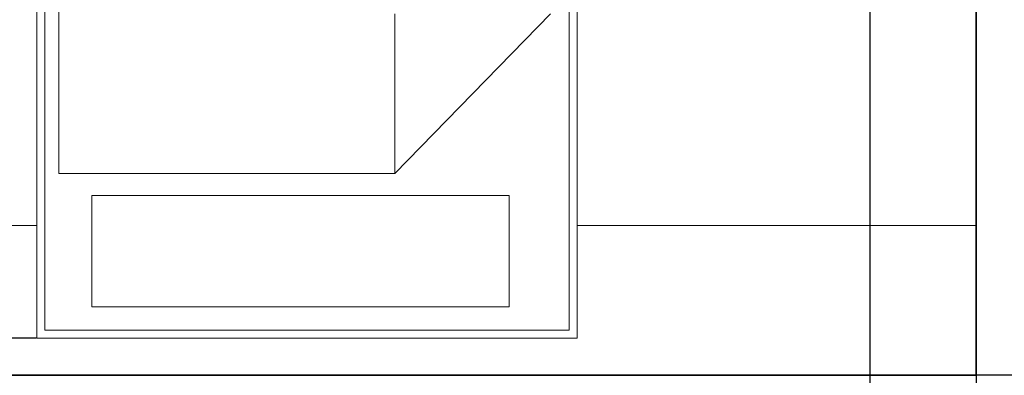
# Model space of a CAD drawing. Units: inches. Extents: x 1291 to 2095, y 532 to 1090.
# Tile 5 of 14: x 1618 to 1696, y 733 to 761. Entities that reach past the tile are written whole.
import ezdxf

# ---------------------------------------------------------------- set-up
doc = ezdxf.new("R2010")
doc.units = ezdxf.units.IN
doc.header["$MEASUREMENT"] = 0
for name, color, linetype, lineweight in [('A-ANNO-DIMS', 2, 'Continuous', 18), ('A-FLOR-CASE', 9, 'Continuous', 18), ('A-FURN', 8, 'Continuous', 18), ('A-WALL', 7, 'Continuous', 35)]:
    doc.layers.add(name, color=color, linetype=linetype, lineweight=lineweight)
doc.styles.get("Standard").update_dxf_attribs({"font": 'arial.ttf'})
doc.dimstyles.get("Standard").update_dxf_attribs({"dimtxt": 4, "dimasz": 0.18, "dimexe": 0.18, "dimexo": 0.0625, "dimgap": 0.09, "dimtad": 0, "dimtih": 1, "dimtoh": 1, "dimdec": 0, "dimrnd": 6, "dimzin": 0, "dimdsep": 46, "dimlunit": 3, "dimtxsty": 'Standard', "dimcen": 0.09, "dimadec": 0, "dimazin": 0, "dimtfac": 1, "dimtdec": 0, "dimtofl": 0, "dimtmove": 0, "dimatfit": 3, "dimfxl": 1, "dimtolj": 1, "dimtzin": 0, "dimarcsym": 0})

# ---------------------------------------------------------------- blocks, each defined once
blk = doc.blocks.new('A$C73B76B3A')
for p, q in [((0, 0), (0, 2)), ((0, 2), (1.35, 2)), ((1.35, 0), (1.35, 2)), ((0.02, 1.98), (1.33, 1.98)), ((0.02, 0.02), (0.02, 1.98)), ((1.33, 1.98), (1.33, 0.02)), ((1.213, 1.9223), (0.1702, 1.9223)), ((0.1702, 1.9223), (0.1702, 1.6438)), ((1.213, 1.6438), (1.213, 1.9223)), ((0.1702, 1.6438), (1.213, 1.6438)), ((0.4562, 1.5889), (0.0673, 1.1899)), ((0.4562, 1.5889), (0.4562, 1.1899)), ((1.2954, 1.5889), (0.4562, 1.5889)), ((1.2954, 0.0644), (1.2954, 1.5889))]:
    blk.add_line(p, q)
blk = doc.blocks.new('*D30')
at = {"layer": 'A-ANNO-DIMS', "color": 0, "lineweight": -2, "transparency": 16777216}
for p, q in [((1618.87, 799.814), (1609.145, 799.814)), ((1609.325, 799.634), (1609.325, 769.922)), ((1609.325, 735.946), (1609.325, 765.658)), ((1618.87, 735.766), (1609.145, 735.766))]:
    blk.add_line(p, q, dxfattribs=at)
at = {"layer": 'A-ANNO-DIMS', "color": 0, "transparency": 16777216}
for points in [[(1609.295, 799.634), (1609.355, 799.634), (1609.325, 799.814)], [(1609.295, 735.946), (1609.355, 735.946), (1609.325, 735.766)]]:
    blk.add_solid(points, dxfattribs=at)
at = {"layer": 'Defpoints', "color": 0, "transparency": 16777216}
for p in [(1618.932, 799.814), (1609.325, 735.766), (1618.932, 735.766)]:
    blk.add_point(p, dxfattribs=at)
at = {"layer": 'A-ANNO-DIMS', "color": 0, "transparency": 16777216, "insert": (1609.325, 767.79), "char_height": 4, "attachment_point": 5}
blk.add_mtext('\\A1;BED 64', dxfattribs=at)
blk = doc.blocks.new('*D46')
at = {"layer": 'A-ANNO-DIMS', "color": 0, "lineweight": -2, "transparency": 16777216}
for p, q in [((1600.27, 579.843), (1600.27, 1087.16)), ((1600.45, 1086.98), (1636.471, 1086.98)), ((1685.404, 1086.98), (1649.383, 1086.98)), ((1685.584, 579.843), (1685.584, 1087.16))]:
    blk.add_line(p, q, dxfattribs=at)
at = {"layer": 'A-ANNO-DIMS', "color": 0, "transparency": 16777216}
for points in [[(1600.45, 1087.01), (1600.45, 1086.95), (1600.27, 1086.98)], [(1685.404, 1087.01), (1685.404, 1086.95), (1685.584, 1086.98)]]:
    blk.add_solid(points, dxfattribs=at)
at = {"layer": 'Defpoints', "color": 0, "transparency": 16777216}
for p in [(1685.584, 1086.98), (1600.27, 579.78), (1685.584, 579.78)]:
    blk.add_point(p, dxfattribs=at)
at = {"layer": 'A-ANNO-DIMS', "color": 0, "transparency": 16777216, "insert": (1642.927, 1086.98), "char_height": 4, "attachment_point": 5}
blk.add_mtext('\\A1;85.31', dxfattribs=at)
blk = doc.blocks.new('*D49')
at = {"layer": 'A-ANNO-DIMS', "color": 0, "lineweight": -2, "transparency": 16777216}
for p, q in [((1694.074, 852.718), (1694.074, 534.4)), ((1586.074, 816.718), (1586.074, 534.4)), ((1586.254, 534.58), (1635.749, 534.58)), ((1693.894, 534.58), (1644.398, 534.58))]:
    blk.add_line(p, q, dxfattribs=at)
at = {"layer": 'A-ANNO-DIMS', "color": 0, "transparency": 16777216}
for points in [[(1586.254, 534.61), (1586.254, 534.55), (1586.074, 534.58)], [(1693.894, 534.61), (1693.894, 534.55), (1694.074, 534.58)]]:
    blk.add_solid(points, dxfattribs=at)
at = {"layer": 'Defpoints', "color": 0, "transparency": 16777216}
for p in [(1694.074, 852.78), (1586.074, 816.78), (1694.074, 534.58)]:
    blk.add_point(p, dxfattribs=at)
at = {"layer": 'A-ANNO-DIMS', "color": 0, "transparency": 16777216, "insert": (1640.074, 534.58), "char_height": 4, "attachment_point": 5}
blk.add_mtext('\\A1;108', dxfattribs=at)
blk = doc.blocks.new('*D51')
at = {"layer": 'A-ANNO-DIMS', "color": 0, "lineweight": -2, "transparency": 16777216}
for p, q in [((1820.011, 852.78), (1297.694, 852.78)), ((1297.874, 852.6), (1297.874, 794.913)), ((1297.874, 732.96), (1297.874, 790.648)), ((1811.011, 732.78), (1297.694, 732.78))]:
    blk.add_line(p, q, dxfattribs=at)
at = {"layer": 'A-ANNO-DIMS', "color": 0, "transparency": 16777216}
for points in [[(1297.844, 852.6), (1297.904, 852.6), (1297.874, 852.78)], [(1297.844, 732.96), (1297.904, 732.96), (1297.874, 732.78)]]:
    blk.add_solid(points, dxfattribs=at)
at = {"layer": 'Defpoints', "color": 0, "transparency": 16777216}
for p in [(1297.874, 852.78), (1820.074, 852.78), (1811.074, 732.78)]:
    blk.add_point(p, dxfattribs=at)
at = {"layer": 'A-ANNO-DIMS', "color": 0, "transparency": 16777216, "insert": (1297.874, 792.78), "char_height": 4, "attachment_point": 5}
blk.add_mtext('\\A1;120', dxfattribs=at)

msp = doc.modelspace()

# ---------------------------------------------------------------- linework, layer by layer
at = {"layer": 'A-FLOR-CASE'}
for p, q in [((1586.0735, 744.7804), (1618.932, 744.7804)), ((1662.1648, 744.7804), (1694.0735, 744.7804))]:
    msp.add_line(p, q, dxfattribs=at)
at = {"layer": 'A-WALL'}
for p, q in [((1694.0735, 732.7804), (1694.0735, 852.7804)), ((1586.0735, 732.7804), (1694.0735, 732.7804))]:
    msp.add_line(p, q, dxfattribs=at)

# ---------------------------------------------------------------- block references
at = {"layer": 'A-FURN', "xscale": 32.02427574694497, "yscale": 32.02427574694497, "zscale": 32.02427574694497, "rotation": 180}
msp.add_blockref('A$C73B76B3A', (1662.1648, 799.8143), dxfattribs=at)

# ---------------------------------------------------------------- dimensions: what is measured, and where the dimension line sits
at = {"layer": 'A-ANNO-DIMS'}
for base, p1, p2, override, picture, middle in [((1685.5842, 1086.9804), (1600.2697, 579.7804), (1685.5842, 579.7804), {"dimdec": 2, "dimlfac": 1, "dimrnd": 0, "dimzin": 0, "dimdsep": 46, "dimlunit": 2}, '*D46', (1642.927, 1086.9804)), ((1694.0735, 534.5804), (1586.0735, 816.7804), (1694.0735, 852.7804), {"dimdec": 0, "dimlfac": 1, "dimrnd": 0, "dimzin": 0, "dimdsep": 46, "dimlunit": 2}, '*D49', (1640.0735, 534.5804))]:
    dim = msp.add_linear_dim(base=base, p1=p1, p2=p2, dimstyle='Standard', override=override, dxfattribs=at)
    dim.commit()
    dim.dimension.update_dxf_attribs({"geometry": picture, "text_midpoint": middle})
dim = msp.add_linear_dim(base=(1297.8735, 852.7804), p1=(1811.0735, 732.7804), p2=(1820.0735, 852.7804), angle=90, dimstyle='Standard', override={"dimdec": 0, "dimlfac": 1, "dimrnd": 0, "dimzin": 0, "dimdsep": 46, "dimlunit": 2}, dxfattribs=at)
dim.commit()
dim.dimension.update_dxf_attribs({"geometry": '*D51', "text_midpoint": (1297.8735, 792.7804)})
dim = msp.add_linear_dim(base=(1609.3247, 735.7658), p1=(1618.932, 799.8143), p2=(1618.932, 735.7658), angle=270, text='BED <>', dimstyle='Standard', override={"dimdec": 0, "dimlfac": 1, "dimrnd": 0, "dimzin": 0, "dimdsep": 46, "dimlunit": 2}, dxfattribs=at)
dim.commit()
dim.dimension.update_dxf_attribs({"geometry": '*D30', "text_midpoint": (1609.3247, 767.79)})

doc.saveas('drawing.dxf')
